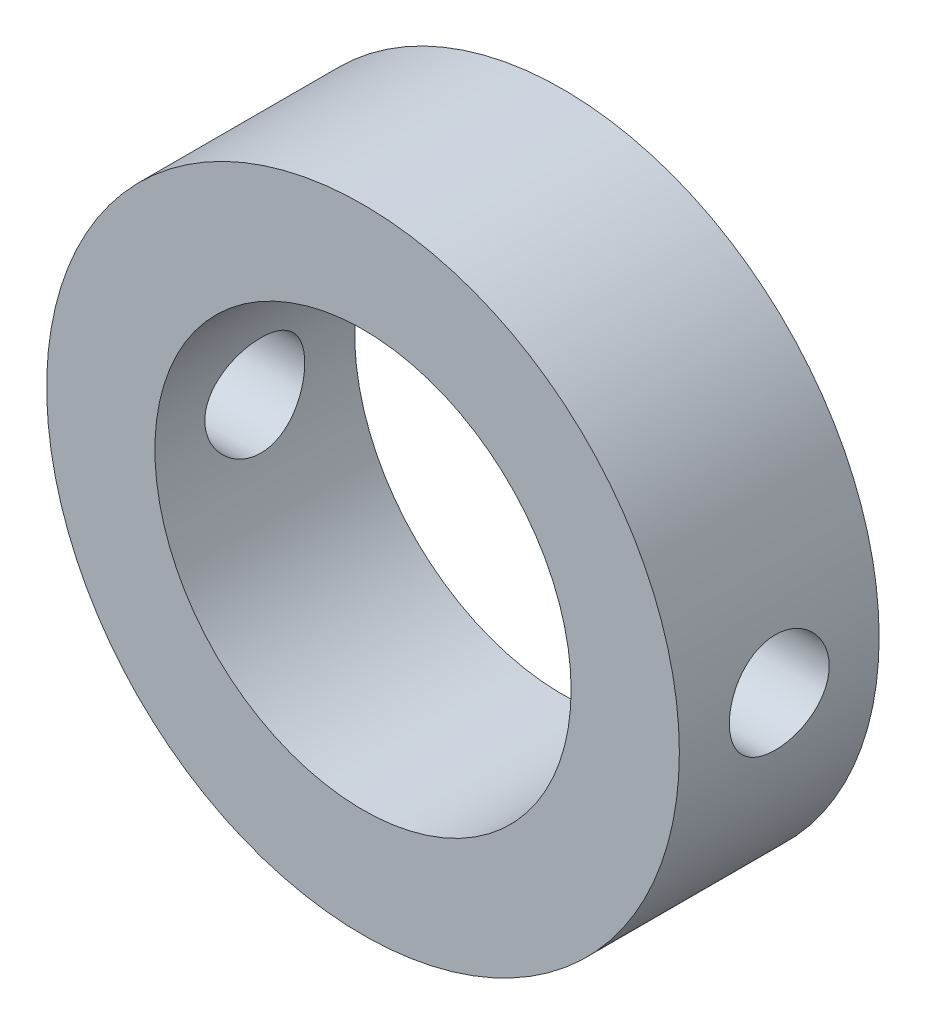
ISO-10303-21;
HEADER;
FILE_DESCRIPTION(('STEP AP214'),'2;1');
FILE_NAME('part.step','',(''),(''),'','','');
FILE_SCHEMA(('AUTOMOTIVE_DESIGN { 1 0 10303 214 1 1 1 1 }'));
ENDSEC;
DATA;
#1=APPLICATION_CONTEXT('core data for automotive mechanical design processes');
#2=APPLICATION_PROTOCOL_DEFINITION('international standard','automotive_design',2000,#1);
#3=PRODUCT_CONTEXT('',#1,'mechanical');
#4=PRODUCT('Part','Part','',(#3));
#5=PRODUCT_RELATED_PRODUCT_CATEGORY('part','',(#4));
#6=PRODUCT_DEFINITION_FORMATION('','',#4);
#7=PRODUCT_DEFINITION_CONTEXT('part definition',#1,'design');
#8=PRODUCT_DEFINITION('design','',#6,#7);
#9=PRODUCT_DEFINITION_SHAPE('','',#8);
#10=(LENGTH_UNIT() NAMED_UNIT(*) SI_UNIT(.MILLI.,.METRE.));
#11=(NAMED_UNIT(*) PLANE_ANGLE_UNIT() SI_UNIT($,.RADIAN.));
#12=(NAMED_UNIT(*) SI_UNIT($,.STERADIAN.) SOLID_ANGLE_UNIT());
#13=UNCERTAINTY_MEASURE_WITH_UNIT(LENGTH_MEASURE(1.E-05),#10,'distance_accuracy_value','');
#14=(GEOMETRIC_REPRESENTATION_CONTEXT(3) GLOBAL_UNCERTAINTY_ASSIGNED_CONTEXT((#13)) GLOBAL_UNIT_ASSIGNED_CONTEXT((#10,
#11,#12)) REPRESENTATION_CONTEXT('',''));
#15=CARTESIAN_POINT('',(0.,0.,0.));
#16=DIRECTION('',(0.,0.,1.));
#17=DIRECTION('',(1.,0.,0.));
#18=AXIS2_PLACEMENT_3D('',#15,#16,#17);
#19=CARTESIAN_POINT('',(0.,0.,12.));
#20=DIRECTION('',(0.,0.,1.));
#21=DIRECTION('',(1.,0.,0.));
#22=AXIS2_PLACEMENT_3D('',#19,#20,#21);
#23=PLANE('',#22);
#24=CARTESIAN_POINT('',(0.,0.,12.));
#25=DIRECTION('',(0.,0.,1.));
#26=DIRECTION('',(1.,0.,0.));
#27=AXIS2_PLACEMENT_3D('',#24,#25,#26);
#28=CIRCLE('',#27,19.);
#29=CARTESIAN_POINT('',(19.,0.,12.));
#30=VERTEX_POINT('',#29);
#31=EDGE_CURVE('E10',#30,#30,#28,.T.);
#32=ORIENTED_EDGE('',*,*,#31,.T.);
#33=EDGE_LOOP('',(#32));
#34=FACE_BOUND('',#33,.T.);
#35=CARTESIAN_POINT('',(0.,0.,12.));
#36=DIRECTION('',(0.,0.,1.));
#37=DIRECTION('',(1.,0.,0.));
#38=AXIS2_PLACEMENT_3D('',#35,#36,#37);
#39=CIRCLE('',#38,12.5);
#40=CARTESIAN_POINT('',(12.5,0.,12.));
#41=VERTEX_POINT('',#40);
#42=EDGE_CURVE('E57',#41,#41,#39,.T.);
#43=ORIENTED_EDGE('',*,*,#42,.F.);
#44=EDGE_LOOP('',(#43));
#45=FACE_BOUND('',#44,.T.);
#46=ADVANCED_FACE('F40',(#34,#45),#23,.T.);
#47=CARTESIAN_POINT('',(0.,0.,0.));
#48=DIRECTION('',(0.,0.,1.));
#49=DIRECTION('',(1.,0.,0.));
#50=AXIS2_PLACEMENT_3D('',#47,#48,#49);
#51=PLANE('',#50);
#52=CARTESIAN_POINT('',(0.,0.,0.));
#53=DIRECTION('',(0.,0.,1.));
#54=DIRECTION('',(1.,0.,0.));
#55=AXIS2_PLACEMENT_3D('',#52,#53,#54);
#56=CIRCLE('',#55,19.);
#57=CARTESIAN_POINT('',(19.,0.,0.));
#58=VERTEX_POINT('',#57);
#59=EDGE_CURVE('E51',#58,#58,#56,.T.);
#60=ORIENTED_EDGE('',*,*,#59,.F.);
#61=EDGE_LOOP('',(#60));
#62=FACE_BOUND('',#61,.T.);
#63=CARTESIAN_POINT('',(0.,0.,0.));
#64=DIRECTION('',(0.,0.,1.));
#65=DIRECTION('',(1.,0.,0.));
#66=AXIS2_PLACEMENT_3D('',#63,#64,#65);
#67=CIRCLE('',#66,12.5);
#68=CARTESIAN_POINT('',(12.5,0.,0.));
#69=VERTEX_POINT('',#68);
#70=EDGE_CURVE('E56',#69,#69,#67,.T.);
#71=ORIENTED_EDGE('',*,*,#70,.T.);
#72=EDGE_LOOP('',(#71));
#73=FACE_BOUND('',#72,.T.);
#74=ADVANCED_FACE('F92',(#62,#73),#51,.F.);
#75=CARTESIAN_POINT('',(0.,0.,12.));
#76=DIRECTION('',(0.,0.,-1.));
#77=DIRECTION('',(-1.,0.,0.));
#78=AXIS2_PLACEMENT_3D('',#75,#76,#77);
#79=CYLINDRICAL_SURFACE('',#78,19.);
#80=CARTESIAN_POINT('',(-19.,0.,3.));
#81=CARTESIAN_POINT('',(-18.9999972240724,0.167395200213042,3.00000681849822));
#82=CARTESIAN_POINT('',(-18.9977646846382,0.334884874788031,3.01405789020566));
#83=CARTESIAN_POINT('',(-18.9890735602357,0.665175270422546,3.06987248693938));
#84=CARTESIAN_POINT('',(-18.9826109658894,0.827971389790521,3.11166230414313));
#85=CARTESIAN_POINT('',(-18.9661853440085,1.14404753345886,3.22166835699392));
#86=CARTESIAN_POINT('',(-18.9562250634571,1.2973349148092,3.28986385866887));
#87=CARTESIAN_POINT('',(-18.9339021624185,1.59026942093823,3.45069309107706));
#88=CARTESIAN_POINT('',(-18.9215398483668,1.72991828221782,3.54332370507908));
#89=CARTESIAN_POINT('',(-18.895666487681,1.99283693302403,3.75124377099957));
#90=CARTESIAN_POINT('',(-18.8821473182235,2.11597212000228,3.86670243752739));
#91=CARTESIAN_POINT('',(-18.8555468666848,2.34120609409226,4.11663696341186));
#92=CARTESIAN_POINT('',(-18.8424656109348,2.44330361812924,4.25111396378837));
#93=CARTESIAN_POINT('',(-18.8181433723965,2.6240952801003,4.53618168893892));
#94=CARTESIAN_POINT('',(-18.8069128876018,2.70265784849317,4.6868568295184));
#95=CARTESIAN_POINT('',(-18.7876755172578,2.83330843623881,4.99947134957592));
#96=CARTESIAN_POINT('',(-18.779668436761,2.88539805669313,5.1614100471529));
#97=CARTESIAN_POINT('',(-18.767864811149,2.96120325071719,5.49053389790333));
#98=CARTESIAN_POINT('',(-18.764033952474,2.98515018535337,5.65766450956719));
#99=CARTESIAN_POINT('',(-18.7609125219047,3.00470725611049,5.99361234611636));
#100=CARTESIAN_POINT('',(-18.7616216614731,3.00031919304727,6.16242946313586));
#101=CARTESIAN_POINT('',(-18.76746874767,2.96351961421685,6.49531594311237));
#102=CARTESIAN_POINT('',(-18.7725658083082,2.93136679776229,6.65941472658318));
#103=CARTESIAN_POINT('',(-18.7865504980478,2.8403558507158,6.97985879214816));
#104=CARTESIAN_POINT('',(-18.79543824493,2.78149689033187,7.13620383315677));
#105=CARTESIAN_POINT('',(-18.8160475867562,2.6384785155272,7.43748362549839));
#106=CARTESIAN_POINT('',(-18.8277813007915,2.55421051731569,7.58236596876211));
#107=CARTESIAN_POINT('',(-18.852751887079,2.3628433457816,7.85603210418096));
#108=CARTESIAN_POINT('',(-18.8659888684252,2.25574251495398,7.98481472653094));
#109=CARTESIAN_POINT('',(-18.8926547085158,2.02033468405641,8.22412423319864));
#110=CARTESIAN_POINT('',(-18.9060840660713,1.89180547305152,8.33443259093931));
#111=CARTESIAN_POINT('',(-18.9314853396994,1.61794401566889,8.53194784285668));
#112=CARTESIAN_POINT('',(-18.943457248079,1.47261168060432,8.61915461509529));
#113=CARTESIAN_POINT('',(-18.9646092293985,1.16907261376921,8.76800642750026));
#114=CARTESIAN_POINT('',(-18.9737873366695,1.01085691624053,8.82963348126301));
#115=CARTESIAN_POINT('',(-18.9883014789364,0.686144192781848,8.92538061400428));
#116=CARTESIAN_POINT('',(-18.9936378020341,0.519647788837095,8.95950275564488));
#117=CARTESIAN_POINT('',(-18.9998286919511,0.184984736062192,8.99897827383141));
#118=CARTESIAN_POINT('',(-19.0007300274,0.0168543348027389,9.0046318768489));
#119=CARTESIAN_POINT('',(-18.9980770575087,-0.317952531425077,8.9878083503127));
#120=CARTESIAN_POINT('',(-18.9945229054864,-0.484629046224455,8.96533218873357));
#121=CARTESIAN_POINT('',(-18.9833872413873,-0.810879134741273,8.89313683736862));
#122=CARTESIAN_POINT('',(-18.9758275205639,-0.970486125590162,8.84356500884154));
#123=CARTESIAN_POINT('',(-18.9575252911701,-1.27912372239425,8.71874166485404));
#124=CARTESIAN_POINT('',(-18.9467826193886,-1.42815378551392,8.64348883252712));
#125=CARTESIAN_POINT('',(-18.9231911639978,-1.71271987736475,8.468743009779));
#126=CARTESIAN_POINT('',(-18.9103262188696,-1.84813841462226,8.36906091242531));
#127=CARTESIAN_POINT('',(-18.883969518103,-2.10043218264525,8.1485479948219));
#128=CARTESIAN_POINT('',(-18.8704777219092,-2.21730621147132,8.02771580482165));
#129=CARTESIAN_POINT('',(-18.8442382720014,-2.43029521840863,7.76699146887425));
#130=CARTESIAN_POINT('',(-18.8314986550647,-2.52620819677151,7.62693337282397));
#131=CARTESIAN_POINT('',(-18.8083518860728,-2.69314533298653,7.33251737546786));
#132=CARTESIAN_POINT('',(-18.7979446657959,-2.76417021883834,7.17815989259932));
#133=CARTESIAN_POINT('',(-18.7807002117535,-2.87900699225531,6.86011177812287));
#134=CARTESIAN_POINT('',(-18.7738493975614,-2.92292252251651,6.69645933767524));
#135=CARTESIAN_POINT('',(-18.7644582567649,-2.98262220399549,6.36398466551931));
#136=CARTESIAN_POINT('',(-18.7619175972673,-2.99840852776725,6.19516283409248));
#137=CARTESIAN_POINT('',(-18.7614477526913,-3.0013458746632,5.85915665401779));
#138=CARTESIAN_POINT('',(-18.7634673948558,-2.98881465767375,5.69197506883905));
#139=CARTESIAN_POINT('',(-18.7717789448073,-2.93615642039242,5.36212973395895));
#140=CARTESIAN_POINT('',(-18.778070842668,-2.89602946421833,5.19946597376149));
#141=CARTESIAN_POINT('',(-18.794199354287,-2.78943553807322,4.88337787030879));
#142=CARTESIAN_POINT('',(-18.804032657621,-2.72299316138579,4.72994505398473));
#143=CARTESIAN_POINT('',(-18.8261396450455,-2.56568649491816,4.43635286334921));
#144=CARTESIAN_POINT('',(-18.8384134296215,-2.47482119948363,4.2961940359378));
#145=CARTESIAN_POINT('',(-18.8641819165768,-2.27010290160429,4.03151806387418));
#146=CARTESIAN_POINT('',(-18.8776882356084,-2.15601525457361,3.90718351682286));
#147=CARTESIAN_POINT('',(-18.9043049971159,-1.90858649068853,3.6793130388949));
#148=CARTESIAN_POINT('',(-18.9174153471904,-1.77524092123377,3.57578193123004));
#149=CARTESIAN_POINT('',(-18.9418556038111,-1.49211329897017,3.391882869579));
#150=CARTESIAN_POINT('',(-18.9531740853537,-1.34223536218178,3.31166102565463));
#151=CARTESIAN_POINT('',(-18.9726437984251,-1.03101937641098,3.17765280690834));
#152=CARTESIAN_POINT('',(-18.9807982506767,-0.86969317979929,3.12383953546548));
#153=CARTESIAN_POINT('',(-18.9911973335544,-0.589739099355738,3.05614181789561));
#154=CARTESIAN_POINT('',(-18.9944810635349,-0.472823930142807,3.03512151616767));
#155=CARTESIAN_POINT('',(-18.9988833649697,-0.237288316828362,3.00704829183149));
#156=CARTESIAN_POINT('',(-19.000001967879,-0.118667897525959,2.99999516630796));
#157=CARTESIAN_POINT('',(-19.,0.,3.));
#158=B_SPLINE_CURVE_WITH_KNOTS('',3,(#80,#81,#82,#83,#84,#85,#86,#87,#88,#89,#90,#91,#92,#93,
#94,#95,#96,#97,#98,#99,#100,#101,#102,#103,#104,#105,#106,#107,#108,#109,#110,#111,#112,#113,
#114,#115,#116,#117,#118,#119,#120,#121,#122,#123,#124,#125,#126,#127,#128,#129,#130,#131,#132,
#133,#134,#135,#136,#137,#138,#139,#140,#141,#142,#143,#144,#145,#146,#147,#148,#149,#150,#151,
#152,#153,#154,#155,#156,#157),.UNSPECIFIED.,.T.,.F.,(4,2,2,2,2,2,2,2,2,2,2,2,2,2,2,2,2,2,2,2,2,
2,2,2,2,2,2,2,2,2,2,2,2,2,2,2,2,2,4),(0.,0.501751911412535,1.00398008893817,1.50581470964933,
2.00758535160925,2.51322514893025,3.01889529538689,3.52734173016572,4.0357574101042,
4.5399634980397,5.04413754173826,5.54366399670822,6.04320597362876,6.54491371515845,
7.04665788959371,7.55397191335254,8.06128861483534,8.56896143470457,9.07659617937734,
9.57886607695304,10.0811186913724,10.5806665697856,11.0802400677869,11.583810193871,
12.0874129449106,12.5956735489114,13.1039192845792,13.6102096956392,14.1164610017594,
14.6170597501047,15.1176573353292,15.6177881828935,16.1179396273336,16.6234208130271,
17.1290190580601,17.6377213704247,18.1459044984556,18.5016059126814,18.8573021592355),.UNSPECIFIED.);
#159=CARTESIAN_POINT('',(-19.,0.,3.));
#160=VERTEX_POINT('',#159);
#161=EDGE_CURVE('E84',#160,#160,#158,.T.);
#162=ORIENTED_EDGE('',*,*,#161,.T.);
#163=EDGE_LOOP('',(#162));
#164=FACE_BOUND('',#163,.T.);
#165=CARTESIAN_POINT('',(19.,0.,3.));
#166=CARTESIAN_POINT('',(18.9999972240724,-0.167395200213042,3.00000681849822));
#167=CARTESIAN_POINT('',(18.9977646846382,-0.334884874788031,3.01405789020566));
#168=CARTESIAN_POINT('',(18.9890735602357,-0.665175270422546,3.06987248693938));
#169=CARTESIAN_POINT('',(18.9826109658894,-0.827971389790521,3.11166230414313));
#170=CARTESIAN_POINT('',(18.9661853440085,-1.14404753345886,3.22166835699392));
#171=CARTESIAN_POINT('',(18.9562250634571,-1.2973349148092,3.28986385866887));
#172=CARTESIAN_POINT('',(18.9339021624185,-1.59026942093823,3.45069309107706));
#173=CARTESIAN_POINT('',(18.9215398483668,-1.72991828221782,3.54332370507908));
#174=CARTESIAN_POINT('',(18.895666487681,-1.99283693302403,3.75124377099957));
#175=CARTESIAN_POINT('',(18.8821473182235,-2.11597212000228,3.86670243752739));
#176=CARTESIAN_POINT('',(18.8555468666848,-2.34120609409226,4.11663696341186));
#177=CARTESIAN_POINT('',(18.8424656109348,-2.44330361812924,4.25111396378837));
#178=CARTESIAN_POINT('',(18.8181433723965,-2.6240952801003,4.53618168893892));
#179=CARTESIAN_POINT('',(18.8069128876018,-2.70265784849317,4.6868568295184));
#180=CARTESIAN_POINT('',(18.7876755172578,-2.83330843623881,4.99947134957592));
#181=CARTESIAN_POINT('',(18.779668436761,-2.88539805669313,5.1614100471529));
#182=CARTESIAN_POINT('',(18.767864811149,-2.96120325071719,5.49053389790333));
#183=CARTESIAN_POINT('',(18.764033952474,-2.98515018535337,5.65766450956719));
#184=CARTESIAN_POINT('',(18.7609125219047,-3.00470725611049,5.99361234611636));
#185=CARTESIAN_POINT('',(18.7616216614731,-3.00031919304727,6.16242946313586));
#186=CARTESIAN_POINT('',(18.76746874767,-2.96351961421685,6.49531594311237));
#187=CARTESIAN_POINT('',(18.7725658083082,-2.93136679776229,6.65941472658318));
#188=CARTESIAN_POINT('',(18.7865504980478,-2.8403558507158,6.97985879214816));
#189=CARTESIAN_POINT('',(18.79543824493,-2.78149689033187,7.13620383315677));
#190=CARTESIAN_POINT('',(18.8160475867562,-2.6384785155272,7.43748362549839));
#191=CARTESIAN_POINT('',(18.8277813007915,-2.55421051731569,7.58236596876211));
#192=CARTESIAN_POINT('',(18.852751887079,-2.3628433457816,7.85603210418096));
#193=CARTESIAN_POINT('',(18.8659888684252,-2.25574251495398,7.98481472653094));
#194=CARTESIAN_POINT('',(18.8926547085158,-2.02033468405641,8.22412423319864));
#195=CARTESIAN_POINT('',(18.9060840660713,-1.89180547305152,8.33443259093931));
#196=CARTESIAN_POINT('',(18.9314853396994,-1.61794401566889,8.53194784285668));
#197=CARTESIAN_POINT('',(18.943457248079,-1.47261168060432,8.61915461509529));
#198=CARTESIAN_POINT('',(18.9646092293985,-1.16907261376921,8.76800642750026));
#199=CARTESIAN_POINT('',(18.9737873366695,-1.01085691624053,8.82963348126301));
#200=CARTESIAN_POINT('',(18.9883014789364,-0.686144192781848,8.92538061400428));
#201=CARTESIAN_POINT('',(18.9936378020341,-0.519647788837095,8.95950275564488));
#202=CARTESIAN_POINT('',(18.9998286919511,-0.184984736062192,8.99897827383141));
#203=CARTESIAN_POINT('',(19.0007300274,-0.0168543348027389,9.0046318768489));
#204=CARTESIAN_POINT('',(18.9980770575087,0.317952531425077,8.9878083503127));
#205=CARTESIAN_POINT('',(18.9945229054864,0.484629046224455,8.96533218873357));
#206=CARTESIAN_POINT('',(18.9833872413873,0.810879134741273,8.89313683736862));
#207=CARTESIAN_POINT('',(18.9758275205639,0.970486125590162,8.84356500884154));
#208=CARTESIAN_POINT('',(18.9575252911701,1.27912372239425,8.71874166485404));
#209=CARTESIAN_POINT('',(18.9467826193886,1.42815378551392,8.64348883252712));
#210=CARTESIAN_POINT('',(18.9231911639978,1.71271987736475,8.468743009779));
#211=CARTESIAN_POINT('',(18.9103262188696,1.84813841462226,8.36906091242531));
#212=CARTESIAN_POINT('',(18.883969518103,2.10043218264525,8.1485479948219));
#213=CARTESIAN_POINT('',(18.8704777219092,2.21730621147132,8.02771580482165));
#214=CARTESIAN_POINT('',(18.8442382720014,2.43029521840863,7.76699146887425));
#215=CARTESIAN_POINT('',(18.8314986550647,2.52620819677151,7.62693337282397));
#216=CARTESIAN_POINT('',(18.8083518860728,2.69314533298653,7.33251737546786));
#217=CARTESIAN_POINT('',(18.7979446657959,2.76417021883834,7.17815989259932));
#218=CARTESIAN_POINT('',(18.7807002117535,2.87900699225531,6.86011177812287));
#219=CARTESIAN_POINT('',(18.7738493975614,2.92292252251651,6.69645933767524));
#220=CARTESIAN_POINT('',(18.7644582567649,2.98262220399549,6.36398466551931));
#221=CARTESIAN_POINT('',(18.7619175972673,2.99840852776725,6.19516283409248));
#222=CARTESIAN_POINT('',(18.7614477526913,3.0013458746632,5.85915665401779));
#223=CARTESIAN_POINT('',(18.7634673948558,2.98881465767375,5.69197506883905));
#224=CARTESIAN_POINT('',(18.7717789448073,2.93615642039242,5.36212973395895));
#225=CARTESIAN_POINT('',(18.778070842668,2.89602946421833,5.19946597376149));
#226=CARTESIAN_POINT('',(18.794199354287,2.78943553807322,4.88337787030879));
#227=CARTESIAN_POINT('',(18.804032657621,2.72299316138579,4.72994505398473));
#228=CARTESIAN_POINT('',(18.8261396450455,2.56568649491816,4.43635286334921));
#229=CARTESIAN_POINT('',(18.8384134296215,2.47482119948363,4.2961940359378));
#230=CARTESIAN_POINT('',(18.8641819165768,2.27010290160429,4.03151806387418));
#231=CARTESIAN_POINT('',(18.8776882356084,2.15601525457361,3.90718351682286));
#232=CARTESIAN_POINT('',(18.9043049971159,1.90858649068853,3.6793130388949));
#233=CARTESIAN_POINT('',(18.9174153471904,1.77524092123377,3.57578193123004));
#234=CARTESIAN_POINT('',(18.9418556038111,1.49211329897017,3.391882869579));
#235=CARTESIAN_POINT('',(18.9531740853537,1.34223536218178,3.31166102565463));
#236=CARTESIAN_POINT('',(18.9726437984251,1.03101937641098,3.17765280690834));
#237=CARTESIAN_POINT('',(18.9807982506767,0.86969317979929,3.12383953546548));
#238=CARTESIAN_POINT('',(18.9911973335544,0.589739099355738,3.05614181789561));
#239=CARTESIAN_POINT('',(18.9944810635349,0.472823930142807,3.03512151616767));
#240=CARTESIAN_POINT('',(18.9988833649697,0.237288316828362,3.00704829183149));
#241=CARTESIAN_POINT('',(19.000001967879,0.118667897525959,2.99999516630796));
#242=CARTESIAN_POINT('',(19.,0.,3.));
#243=B_SPLINE_CURVE_WITH_KNOTS('',3,(#165,#166,#167,#168,#169,#170,#171,#172,#173,#174,#175,
#176,#177,#178,#179,#180,#181,#182,#183,#184,#185,#186,#187,#188,#189,#190,#191,#192,#193,#194,
#195,#196,#197,#198,#199,#200,#201,#202,#203,#204,#205,#206,#207,#208,#209,#210,#211,#212,#213,
#214,#215,#216,#217,#218,#219,#220,#221,#222,#223,#224,#225,#226,#227,#228,#229,#230,#231,#232,
#233,#234,#235,#236,#237,#238,#239,#240,#241,#242),.UNSPECIFIED.,.T.,.F.,(4,2,2,2,2,2,2,2,2,2,2,
2,2,2,2,2,2,2,2,2,2,2,2,2,2,2,2,2,2,2,2,2,2,2,2,2,2,2,4),(0.,0.501751911412535,1.00398008893817,
1.50581470964933,2.00758535160925,2.51322514893025,3.01889529538689,3.52734173016572,
4.0357574101042,4.5399634980397,5.04413754173826,5.54366399670822,6.04320597362876,
6.54491371515845,7.04665788959371,7.55397191335254,8.06128861483534,8.56896143470457,
9.07659617937734,9.57886607695304,10.0811186913724,10.5806665697856,11.0802400677869,
11.583810193871,12.0874129449106,12.5956735489114,13.1039192845792,13.6102096956392,
14.1164610017594,14.6170597501047,15.1176573353292,15.6177881828935,16.1179396273336,
16.6234208130271,17.1290190580601,17.6377213704247,18.1459044984556,18.5016059126814,
18.8573021592355),.UNSPECIFIED.);
#244=CARTESIAN_POINT('',(19.,0.,3.));
#245=VERTEX_POINT('',#244);
#246=EDGE_CURVE('E76',#245,#245,#243,.T.);
#247=ORIENTED_EDGE('',*,*,#246,.T.);
#248=EDGE_LOOP('',(#247));
#249=FACE_BOUND('',#248,.T.);
#250=ORIENTED_EDGE('',*,*,#31,.F.);
#251=EDGE_LOOP('',(#250));
#252=FACE_BOUND('',#251,.T.);
#253=ORIENTED_EDGE('',*,*,#59,.T.);
#254=EDGE_LOOP('',(#253));
#255=FACE_BOUND('',#254,.T.);
#256=ADVANCED_FACE('F39',(#164,#249,#252,#255),#79,.T.);
#257=CARTESIAN_POINT('',(0.,0.,12.));
#258=DIRECTION('',(0.,0.,-1.));
#259=DIRECTION('',(-1.,0.,0.));
#260=AXIS2_PLACEMENT_3D('',#257,#258,#259);
#261=CYLINDRICAL_SURFACE('',#260,12.5);
#262=CARTESIAN_POINT('',(-12.5,0.,9.00000000000001));
#263=CARTESIAN_POINT('',(-12.4999970714968,-0.165963929028716,8.99999497592274));
#264=CARTESIAN_POINT('',(-12.4966615634859,-0.331985420928068,8.98618158976393));
#265=CARTESIAN_POINT('',(-12.4836783946933,-0.65928429097138,8.93136726040463));
#266=CARTESIAN_POINT('',(-12.4740268462166,-0.820558683214275,8.89034957200533));
#267=CARTESIAN_POINT('',(-12.4494823208195,-1.13358839471402,8.78250766549565));
#268=CARTESIAN_POINT('',(-12.4345953702841,-1.28535442324822,8.71571311014241));
#269=CARTESIAN_POINT('',(-12.4011725442513,-1.57552517879763,8.55831456355411));
#270=CARTESIAN_POINT('',(-12.3826366165873,-1.71392971475166,8.46771023192274));
#271=CARTESIAN_POINT('',(-12.3435386014785,-1.97609263393972,8.26343582162448));
#272=CARTESIAN_POINT('',(-12.3229472454311,-2.0995595210048,8.14939721895075));
#273=CARTESIAN_POINT('',(-12.2822574370147,-2.32581080811943,7.90228113093536));
#274=CARTESIAN_POINT('',(-12.2621590363612,-2.42859304624489,7.76920165795906));
#275=CARTESIAN_POINT('',(-12.224437969062,-2.61189993555015,7.48555416698255));
#276=CARTESIAN_POINT('',(-12.2068525815312,-2.69210377047565,7.33477341624116));
#277=CARTESIAN_POINT('',(-12.1765733412448,-2.82591582947333,7.02138016487152));
#278=CARTESIAN_POINT('',(-12.1638787734309,-2.87952794169564,6.85876939797685));
#279=CARTESIAN_POINT('',(-12.1451184675007,-2.95765058108663,6.5295234267311));
#280=CARTESIAN_POINT('',(-12.1389341034343,-2.98268262400616,6.3630188784745));
#281=CARTESIAN_POINT('',(-12.1335389605945,-3.00455808879087,6.02806762035725));
#282=CARTESIAN_POINT('',(-12.1343271412568,-3.00140571682399,5.85962120404308));
#283=CARTESIAN_POINT('',(-12.1426811387008,-2.96741912081942,5.52952403398712));
#284=CARTESIAN_POINT('',(-12.1500960921292,-2.93720103400494,5.36780543481045));
#285=CARTESIAN_POINT('',(-12.1706283738785,-2.85092141637189,5.05180268335217));
#286=CARTESIAN_POINT('',(-12.1837460799133,-2.79485817372027,4.89751902426558));
#287=CARTESIAN_POINT('',(-12.2143476734445,-2.65794121231782,4.59908702191565));
#288=CARTESIAN_POINT('',(-12.2318714325758,-2.5768594824696,4.45504754708331));
#289=CARTESIAN_POINT('',(-12.2692875046197,-2.39236688956383,4.18239549927743));
#290=CARTESIAN_POINT('',(-12.2891802016137,-2.28895240342647,4.05378543471489));
#291=CARTESIAN_POINT('',(-12.329732025739,-2.05951493908847,3.81210642968127));
#292=CARTESIAN_POINT('',(-12.3503975788014,-1.93297064389908,3.69953290093779));
#293=CARTESIAN_POINT('',(-12.3896951594929,-1.66255592459692,3.49711528025362));
#294=CARTESIAN_POINT('',(-12.4083271342049,-1.51868504982141,3.40727177970739));
#295=CARTESIAN_POINT('',(-12.4415394956922,-1.21702847718581,3.25270277938723));
#296=CARTESIAN_POINT('',(-12.4561077058019,-1.05920278696054,3.18805254376222));
#297=CARTESIAN_POINT('',(-12.4794620474154,-0.734497606078677,3.08633492095142));
#298=CARTESIAN_POINT('',(-12.4882491958651,-0.567619713387662,3.04926268237319));
#299=CARTESIAN_POINT('',(-12.4989027542709,-0.233787399651665,3.00449793534797));
#300=CARTESIAN_POINT('',(-12.5009282130753,-0.0669284805450082,2.99613010753843));
#301=CARTESIAN_POINT('',(-12.4982807419474,0.265804381586629,3.00716676685091));
#302=CARTESIAN_POINT('',(-12.4936083648176,0.431678404764952,3.02656896198724));
#303=CARTESIAN_POINT('',(-12.4781916395217,0.755422580108847,3.09203697851639));
#304=CARTESIAN_POINT('',(-12.4675301590363,0.913370579311303,3.13773910957381));
#305=CARTESIAN_POINT('',(-12.4413335015664,1.21935330013476,3.25409819169527));
#306=CARTESIAN_POINT('',(-12.4257978558334,1.3673870666415,3.32475754297811));
#307=CARTESIAN_POINT('',(-12.3911910149582,1.6520615099557,3.49036659359786));
#308=CARTESIAN_POINT('',(-12.3720653178033,1.78847176740355,3.58570071692438));
#309=CARTESIAN_POINT('',(-12.3324936406987,2.04359904096632,3.79745692901342));
#310=CARTESIAN_POINT('',(-12.3120474520734,2.16231325074337,3.91388235608078));
#311=CARTESIAN_POINT('',(-12.2715742142771,2.38142453789941,4.16764083120856));
#312=CARTESIAN_POINT('',(-12.2515669262668,2.4813497404737,4.30538512208211));
#313=CARTESIAN_POINT('',(-12.2147538797452,2.65666020824081,4.59609042789674));
#314=CARTESIAN_POINT('',(-12.1979479778962,2.7320465722335,4.74905076109348));
#315=CARTESIAN_POINT('',(-12.1696189519335,2.85558993518171,5.06501251354399));
#316=CARTESIAN_POINT('',(-12.1580647463107,2.90390754385905,5.22794820342123));
#317=CARTESIAN_POINT('',(-12.1415072663683,2.97238380283979,5.5599461850207));
#318=CARTESIAN_POINT('',(-12.1365026916888,2.99254804274991,5.72900725376178));
#319=CARTESIAN_POINT('',(-12.1337046220624,3.00387066449353,6.0636707002806));
#320=CARTESIAN_POINT('',(-12.1357241633848,2.99578106592266,6.2292464963267));
#321=CARTESIAN_POINT('',(-12.1463176460425,2.95253345626267,6.5565997642237));
#322=CARTESIAN_POINT('',(-12.1548914750658,2.91737590900096,6.71837730111136));
#323=CARTESIAN_POINT('',(-12.1775274976748,2.82138591303537,7.03279755254825));
#324=CARTESIAN_POINT('',(-12.191561756094,2.76068402045612,7.18548227258376));
#325=CARTESIAN_POINT('',(-12.2235433612686,2.61543373580583,7.47860441388369));
#326=CARTESIAN_POINT('',(-12.2414912075257,2.53088229934855,7.61904026858636));
#327=CARTESIAN_POINT('',(-12.279819325529,2.33793007708464,7.88733700011951));
#328=CARTESIAN_POINT('',(-12.3002478697533,2.22900267979018,8.01481232309873));
#329=CARTESIAN_POINT('',(-12.3409359831145,1.99143074773236,8.24991998805193));
#330=CARTESIAN_POINT('',(-12.361195511444,1.86278158874234,8.35754766321025));
#331=CARTESIAN_POINT('',(-12.3996570299581,1.5868829988014,8.55160925955475));
#332=CARTESIAN_POINT('',(-12.4178200201219,1.43936414359402,8.63766840544201));
#333=CARTESIAN_POINT('',(-12.4496380610582,1.13153622828567,8.7836295327479));
#334=CARTESIAN_POINT('',(-12.4632965272855,0.971236973691221,8.84355134339162));
#335=CARTESIAN_POINT('',(-12.4824059901497,0.675887025694766,8.9260386251378));
#336=CARTESIAN_POINT('',(-12.4889599449579,0.542312066268421,8.95371661578571));
#337=CARTESIAN_POINT('',(-12.4977580149525,0.272504227478249,8.99069878085188));
#338=CARTESIAN_POINT('',(-12.5000024045682,0.136271517915777,9.00000412522552));
#339=CARTESIAN_POINT('',(-12.5,0.,9.00000000000001));
#340=B_SPLINE_CURVE_WITH_KNOTS('',3,(#262,#263,#264,#265,#266,#267,#268,#269,#270,#271,#272,
#273,#274,#275,#276,#277,#278,#279,#280,#281,#282,#283,#284,#285,#286,#287,#288,#289,#290,#291,
#292,#293,#294,#295,#296,#297,#298,#299,#300,#301,#302,#303,#304,#305,#306,#307,#308,#309,#310,
#311,#312,#313,#314,#315,#316,#317,#318,#319,#320,#321,#322,#323,#324,#325,#326,#327,#328,#329,
#330,#331,#332,#333,#334,#335,#336,#337,#338,#339),.UNSPECIFIED.,.T.,.F.,(4,2,2,2,2,2,2,2,2,2,2,
2,2,2,2,2,2,2,2,2,2,2,2,2,2,2,2,2,2,2,2,2,2,2,2,2,2,2,4),(0.,0.497392599366679,
0.995091645758824,1.49221966408501,1.98935478998519,2.49500570148357,3.00070943533306,
3.51327262050849,4.02576083835037,4.5287399535911,5.03164400680465,5.52338274964838,
6.01515406709138,6.51154667521171,7.00801987450003,7.51749958381934,8.0269925475217,
8.53799614678203,9.04890983140415,9.54771776810826,10.0464845383097,10.5385143736981,
11.0305915421211,11.5308523313794,12.031192370573,12.5427824523192,13.0543496229377,
13.5628484119093,14.0712462285018,14.5662165454702,15.0611783809799,15.5536406351284,
16.0461657803879,16.5505844610431,17.0551215958269,17.5678974206352,18.0802835459069,
18.4887142303991,18.897118905514),.UNSPECIFIED.);
#341=CARTESIAN_POINT('',(-12.5,0.,9.00000000000001));
#342=VERTEX_POINT('',#341);
#343=EDGE_CURVE('E45',#342,#342,#340,.T.);
#344=ORIENTED_EDGE('',*,*,#343,.F.);
#345=EDGE_LOOP('',(#344));
#346=FACE_BOUND('',#345,.T.);
#347=CARTESIAN_POINT('',(12.5,0.,3.));
#348=CARTESIAN_POINT('',(12.4999970714968,-0.165963929028716,3.00000502407727));
#349=CARTESIAN_POINT('',(12.4966615634859,-0.331985420928068,3.01381841023608));
#350=CARTESIAN_POINT('',(12.4836783946933,-0.65928429097138,3.06863273959538));
#351=CARTESIAN_POINT('',(12.4740268462166,-0.820558683214275,3.10965042799468));
#352=CARTESIAN_POINT('',(12.4494823208195,-1.13358839471402,3.21749233450436));
#353=CARTESIAN_POINT('',(12.4345953702841,-1.28535442324822,3.2842868898576));
#354=CARTESIAN_POINT('',(12.4011725442513,-1.57552517879763,3.4416854364459));
#355=CARTESIAN_POINT('',(12.3826366165873,-1.71392971475166,3.53228976807727));
#356=CARTESIAN_POINT('',(12.3435386014785,-1.97609263393972,3.73656417837553));
#357=CARTESIAN_POINT('',(12.3229472454311,-2.0995595210048,3.85060278104927));
#358=CARTESIAN_POINT('',(12.2822574370147,-2.32581080811943,4.09771886906465));
#359=CARTESIAN_POINT('',(12.2621590363612,-2.42859304624489,4.23079834204096));
#360=CARTESIAN_POINT('',(12.224437969062,-2.61189993555015,4.51444583301746));
#361=CARTESIAN_POINT('',(12.2068525815312,-2.69210377047565,4.66522658375885));
#362=CARTESIAN_POINT('',(12.1765733412448,-2.82591582947332,4.97861983512849));
#363=CARTESIAN_POINT('',(12.1638787734309,-2.87952794169564,5.14123060202316));
#364=CARTESIAN_POINT('',(12.1451184675007,-2.95765058108663,5.47047657326891));
#365=CARTESIAN_POINT('',(12.1389341034343,-2.98268262400616,5.63698112152551));
#366=CARTESIAN_POINT('',(12.1335389605945,-3.00455808879087,5.97193237964276));
#367=CARTESIAN_POINT('',(12.1343271412568,-3.00140571682399,6.14037879595693));
#368=CARTESIAN_POINT('',(12.1426811387008,-2.96741912081942,6.47047596601289));
#369=CARTESIAN_POINT('',(12.1500960921292,-2.93720103400494,6.63219456518956));
#370=CARTESIAN_POINT('',(12.1706283738785,-2.85092141637189,6.94819731664784));
#371=CARTESIAN_POINT('',(12.1837460799133,-2.79485817372027,7.10248097573443));
#372=CARTESIAN_POINT('',(12.2143476734445,-2.65794121231782,7.40091297808436));
#373=CARTESIAN_POINT('',(12.2318714325758,-2.5768594824696,7.5449524529167));
#374=CARTESIAN_POINT('',(12.2692875046197,-2.39236688956383,7.81760450072258));
#375=CARTESIAN_POINT('',(12.2891802016137,-2.28895240342647,7.94621456528511));
#376=CARTESIAN_POINT('',(12.329732025739,-2.05951493908847,8.18789357031874));
#377=CARTESIAN_POINT('',(12.3503975788014,-1.93297064389908,8.30046709906222));
#378=CARTESIAN_POINT('',(12.3896951594929,-1.66255592459692,8.50288471974639));
#379=CARTESIAN_POINT('',(12.4083271342049,-1.51868504982141,8.59272822029262));
#380=CARTESIAN_POINT('',(12.4415394956922,-1.21702847718581,8.74729722061278));
#381=CARTESIAN_POINT('',(12.4561077058019,-1.05920278696054,8.81194745623779));
#382=CARTESIAN_POINT('',(12.4794620474154,-0.734497606078676,8.91366507904859));
#383=CARTESIAN_POINT('',(12.4882491958651,-0.567619713387662,8.95073731762682));
#384=CARTESIAN_POINT('',(12.4989027542709,-0.233787399651664,8.99550206465204));
#385=CARTESIAN_POINT('',(12.5009282130753,-0.0669284805450071,9.00386989246158));
#386=CARTESIAN_POINT('',(12.4982807419474,0.26580438158663,8.9928332331491));
#387=CARTESIAN_POINT('',(12.4936083648176,0.431678404764953,8.97343103801277));
#388=CARTESIAN_POINT('',(12.4781916395217,0.755422580108846,8.90796302148362));
#389=CARTESIAN_POINT('',(12.4675301590363,0.913370579311301,8.8622608904262));
#390=CARTESIAN_POINT('',(12.4413335015664,1.21935330013476,8.74590180830474));
#391=CARTESIAN_POINT('',(12.4257978558334,1.3673870666415,8.6752424570219));
#392=CARTESIAN_POINT('',(12.3911910149582,1.6520615099557,8.50963340640215));
#393=CARTESIAN_POINT('',(12.3720653178033,1.78847176740355,8.41429928307563));
#394=CARTESIAN_POINT('',(12.3324936406987,2.04359904096632,8.20254307098659));
#395=CARTESIAN_POINT('',(12.3120474520734,2.16231325074336,8.08611764391923));
#396=CARTESIAN_POINT('',(12.2715742142771,2.38142453789941,7.83235916879145));
#397=CARTESIAN_POINT('',(12.2515669262668,2.4813497404737,7.6946148779179));
#398=CARTESIAN_POINT('',(12.2147538797452,2.65666020824081,7.40390957210327));
#399=CARTESIAN_POINT('',(12.1979479778962,2.7320465722335,7.25094923890653));
#400=CARTESIAN_POINT('',(12.1696189519335,2.85558993518171,6.93498748645602));
#401=CARTESIAN_POINT('',(12.1580647463107,2.90390754385905,6.77205179657878));
#402=CARTESIAN_POINT('',(12.1415072663683,2.97238380283979,6.44005381497931));
#403=CARTESIAN_POINT('',(12.1365026916888,2.99254804274991,6.27099274623823));
#404=CARTESIAN_POINT('',(12.1337046220624,3.00387066449353,5.93632929971941));
#405=CARTESIAN_POINT('',(12.1357241633848,2.99578106592266,5.77075350367331));
#406=CARTESIAN_POINT('',(12.1463176460425,2.95253345626267,5.44340023577631));
#407=CARTESIAN_POINT('',(12.1548914750658,2.91737590900096,5.28162269888865));
#408=CARTESIAN_POINT('',(12.1775274976748,2.82138591303537,4.96720244745176));
#409=CARTESIAN_POINT('',(12.191561756094,2.76068402045612,4.81451772741625));
#410=CARTESIAN_POINT('',(12.2235433612686,2.61543373580582,4.52139558611631));
#411=CARTESIAN_POINT('',(12.2414912075257,2.53088229934855,4.38095973141365));
#412=CARTESIAN_POINT('',(12.279819325529,2.33793007708464,4.1126629998805));
#413=CARTESIAN_POINT('',(12.3002478697533,2.22900267979018,3.98518767690128));
#414=CARTESIAN_POINT('',(12.3409359831145,1.99143074773236,3.75008001194808));
#415=CARTESIAN_POINT('',(12.361195511444,1.86278158874234,3.64245233678976));
#416=CARTESIAN_POINT('',(12.3996570299581,1.5868829988014,3.44839074044526));
#417=CARTESIAN_POINT('',(12.4178200201219,1.43936414359402,3.362331594558));
#418=CARTESIAN_POINT('',(12.4496380610582,1.13153622828567,3.21637046725211));
#419=CARTESIAN_POINT('',(12.4632965272855,0.971236973691219,3.15644865660839));
#420=CARTESIAN_POINT('',(12.4824059901497,0.675887025694765,3.07396137486221));
#421=CARTESIAN_POINT('',(12.4889599449579,0.542312066268421,3.0462833842143));
#422=CARTESIAN_POINT('',(12.4977580149525,0.272504227478249,3.00930121914813));
#423=CARTESIAN_POINT('',(12.5000024045682,0.136271517915777,2.99999587477449));
#424=CARTESIAN_POINT('',(12.5,0.,3.));
#425=B_SPLINE_CURVE_WITH_KNOTS('',3,(#347,#348,#349,#350,#351,#352,#353,#354,#355,#356,#357,
#358,#359,#360,#361,#362,#363,#364,#365,#366,#367,#368,#369,#370,#371,#372,#373,#374,#375,#376,
#377,#378,#379,#380,#381,#382,#383,#384,#385,#386,#387,#388,#389,#390,#391,#392,#393,#394,#395,
#396,#397,#398,#399,#400,#401,#402,#403,#404,#405,#406,#407,#408,#409,#410,#411,#412,#413,#414,
#415,#416,#417,#418,#419,#420,#421,#422,#423,#424),.UNSPECIFIED.,.T.,.F.,(4,2,2,2,2,2,2,2,2,2,2,
2,2,2,2,2,2,2,2,2,2,2,2,2,2,2,2,2,2,2,2,2,2,2,2,2,2,2,4),(0.,0.497392599366679,
0.995091645758824,1.49221966408501,1.98935478998519,2.49500570148357,3.00070943533306,
3.51327262050849,4.02576083835037,4.52873995359111,5.03164400680465,5.52338274964838,
6.01515406709138,6.51154667521171,7.00801987450003,7.51749958381934,8.0269925475217,
8.53799614678203,9.04890983140415,9.54771776810826,10.0464845383097,10.5385143736981,
11.0305915421211,11.5308523313794,12.031192370573,12.5427824523192,13.0543496229377,
13.5628484119093,14.0712462285018,14.5662165454702,15.0611783809799,15.5536406351284,
16.0461657803879,16.5505844610431,17.0551215958269,17.5678974206352,18.0802835459069,
18.4887142303991,18.897118905514),.UNSPECIFIED.);
#426=CARTESIAN_POINT('',(12.5,0.,3.));
#427=VERTEX_POINT('',#426);
#428=EDGE_CURVE('E62',#427,#427,#425,.T.);
#429=ORIENTED_EDGE('',*,*,#428,.F.);
#430=EDGE_LOOP('',(#429));
#431=FACE_BOUND('',#430,.T.);
#432=ORIENTED_EDGE('',*,*,#42,.T.);
#433=EDGE_LOOP('',(#432));
#434=FACE_BOUND('',#433,.T.);
#435=ORIENTED_EDGE('',*,*,#70,.F.);
#436=EDGE_LOOP('',(#435));
#437=FACE_BOUND('',#436,.T.);
#438=ADVANCED_FACE('F67',(#346,#431,#434,#437),#261,.F.);
#439=CARTESIAN_POINT('',(-19.,0.,6.00000000000001));
#440=DIRECTION('',(1.,0.,0.));
#441=DIRECTION('',(0.,0.,-1.));
#442=AXIS2_PLACEMENT_3D('',#439,#440,#441);
#443=CYLINDRICAL_SURFACE('',#442,3.);
#444=ORIENTED_EDGE('',*,*,#428,.T.);
#445=EDGE_LOOP('',(#444));
#446=FACE_BOUND('',#445,.T.);
#447=ORIENTED_EDGE('',*,*,#246,.F.);
#448=EDGE_LOOP('',(#447));
#449=FACE_BOUND('',#448,.T.);
#450=ADVANCED_FACE('F75',(#446,#449),#443,.F.);
#451=ORIENTED_EDGE('',*,*,#343,.T.);
#452=EDGE_LOOP('',(#451));
#453=FACE_BOUND('',#452,.T.);
#454=ORIENTED_EDGE('',*,*,#161,.F.);
#455=EDGE_LOOP('',(#454));
#456=FACE_BOUND('',#455,.T.);
#457=ADVANCED_FACE('F69',(#453,#456),#443,.F.);
#458=CLOSED_SHELL('',(#46,#74,#256,#438,#450,#457));
#459=MANIFOLD_SOLID_BREP('B2',#458);
#460=ADVANCED_BREP_SHAPE_REPRESENTATION('',(#18,#459),#14);
#461=SHAPE_DEFINITION_REPRESENTATION(#9,#460);
ENDSEC;
END-ISO-10303-21;
